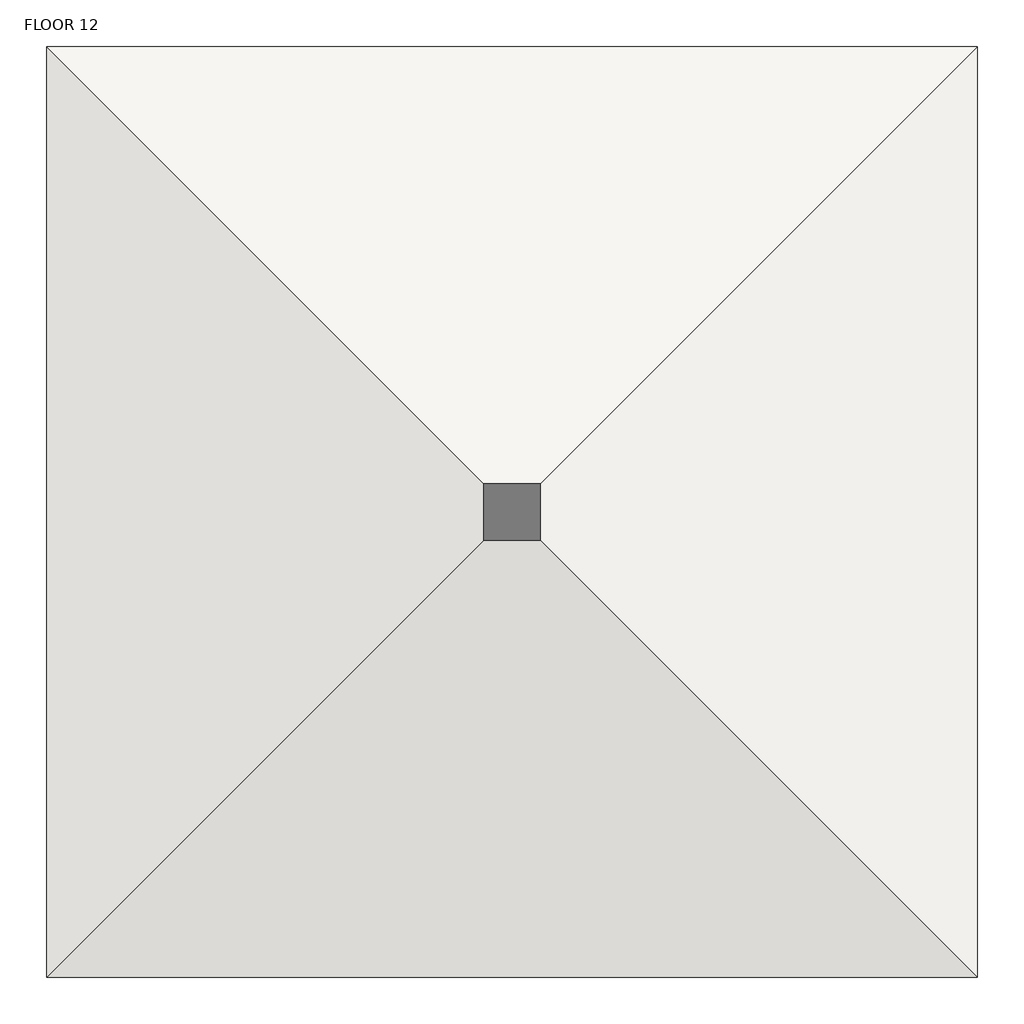
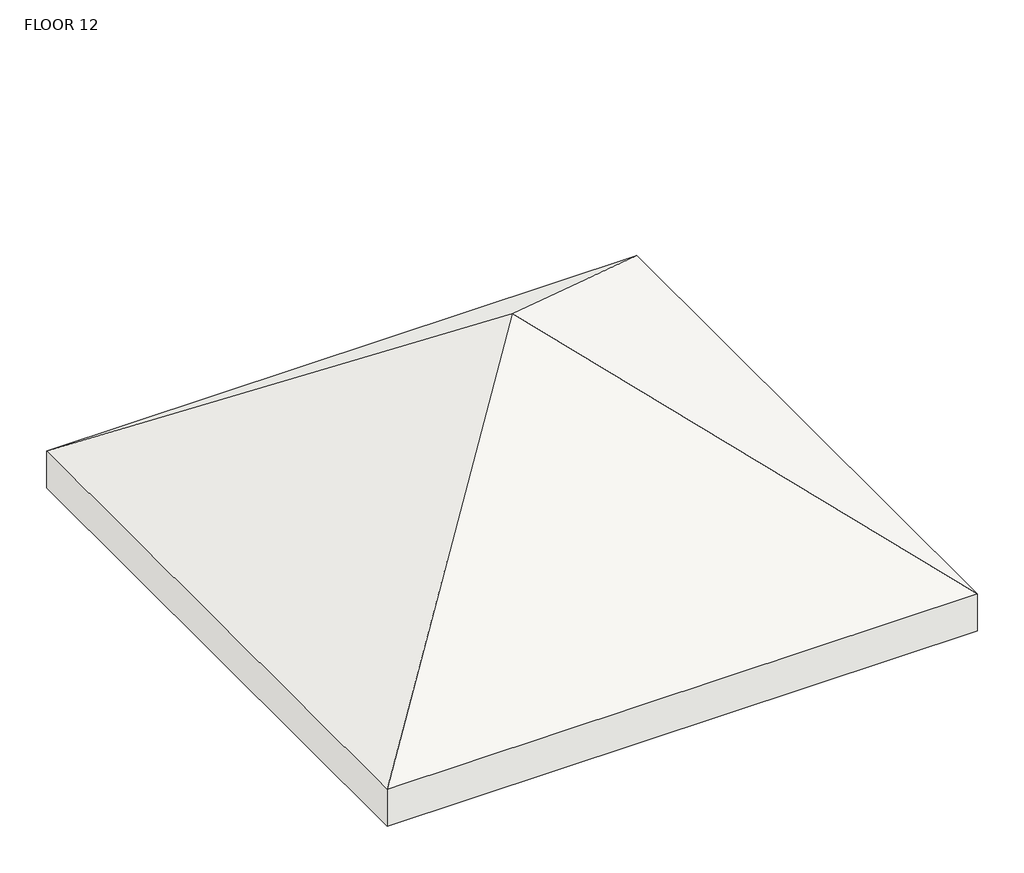
# One storey: 1 roof.
"""IFC4 building model written with IfcOpenShell, lengths in millimetres."""

from ifc_helpers import new_model, si_unit, origin, place, context, project, spatial, faceted_brep, element, save

model = new_model("IFC4")

# Units and contexts
model_context = context("Model", 3, world=origin())
ifc_project = project(units=[si_unit("LENGTHUNIT", "METRE", prefix="MILLI")], contexts=[model_context])

# Site, building, storey
site = spatial("IfcSite", under=ifc_project)
building = spatial("IfcBuilding", under=site)
storey = spatial("IfcBuildingStorey", under=building, Name="FLOOR 12", Elevation=18078.7725604)

# Roof
placement = place(None, origin())
element("IfcRoof", 1, ObjectType="Generic - 12\"", at=placement, inside=storey, context=model_context, shape_type="Brep", body=[
    faceted_brep([(-3481.6094527, -3246.5242565, 18078.7725604), (-4916.7094527, -4681.6242565, 19155.0975604), (-6351.8094527, -3246.5242565, 18078.7725604), (-6351.8094527, -6116.7242565, 18078.7725604), (-3481.6094527, -6116.7242565, 18078.7725604), (-3481.6094527, -3246.5242565, 18269.2725604), (-6351.8094527, -3246.5242565, 18269.2725604), (-4916.7094527, -4681.6242565, 19345.5975604), (-6351.8094527, -6116.7242565, 18269.2725604), (-3481.6094527, -6116.7242565, 18269.2725604)], [[[0, 1, 2]], [[2, 1, 3]], [[3, 1, 4]], [[1, 0, 4]], [[5, 6, 7]], [[6, 8, 7]], [[8, 9, 7]], [[5, 7, 9]], [[2, 6, 5, 0]], [[3, 8, 6, 2]], [[4, 9, 8, 3]], [[0, 5, 9, 4]]]),
])

save(model, "model.ifc")

# Revit data of these elements
# Type "Generic - 12\""
#   Assembly Code = "B1020"
#   Layers, outside or top first: 0' - 6" no material (function 1)
# Element 1 (IfcRoof, "Generic - 12\"")
#   built-in parameter 1001705 = 63.4698 (stored number, unit not read)
#   built-in parameter 1001710 = 33615
#   Phase Created = New Construction
#   Materials on its faces: "Default Roof"
# Materials
#   "Default Roof": colour RGB 88 101 114, transparency 0, Cost = 0
